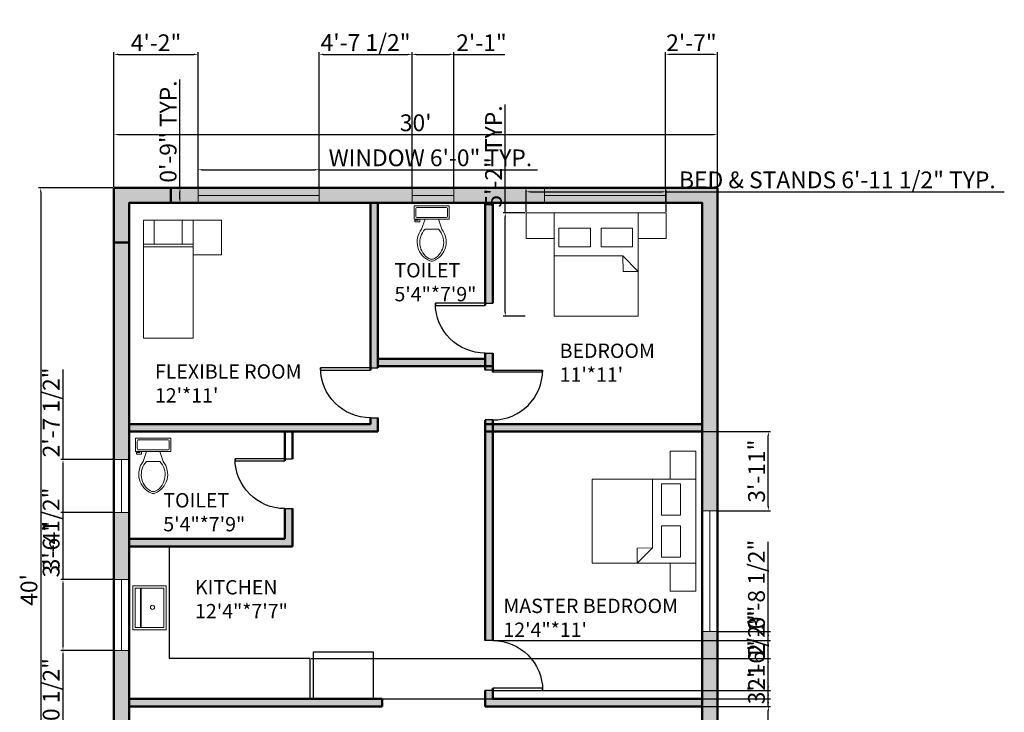
# Model space of a CAD drawing. Units: inches. Extents: x 1369 to 1956, y 3714 to 4363.
# Tile 2 of 2: x 1369 to 1956, y 3949 to 4363. Entities that reach past the tile are written whole.
import ezdxf

# ---------------------------------------------------------------- set-up
doc = ezdxf.new("R2010")
doc.units = ezdxf.units.IN
for name, color, linetype, lineweight in [('A-ANNO-DIMS', 2, 'Continuous', 18), ('A-AREA-IDEN', 7, 'Continuous', 25), ('A-DOOR', 3, 'Continuous', 25), ('A-FLOR-CASE', 9, 'Continuous', 25), ('A-FLOR-FIXT', 9, 'Continuous', 18), ('A-FURN', 8, 'Continuous', 18), ('A-GLAZ', 4, 'Continuous', 18), ('A-WALL', 7, 'Continuous', 50), ('A-WALL-PATT', 252, 'Continuous', 13)]:
    doc.layers.add(name, color=color, linetype=linetype, lineweight=lineweight)
doc.styles.get("Standard").update_dxf_attribs({"font": 'arial.ttf'})
doc.dimstyles.new('ISO-25', dxfattribs={"dimtxt": 10, "dimasz": 2.5, "dimexe": 1.25, "dimexo": 0.625, "dimtad": 1, "dimdec": 0, "dimlunit": 4, "dimtxsty": 'Standard', "dimcen": 2.5, "dimadec": 0, "dimazin": 0, "dimtfac": 1, "dimtdec": 0, "dimtmove": 0, "dimatfit": 3, "dimfxl": 1, "dimarcsym": 0})

# ---------------------------------------------------------------- blocks, each defined once
blk = doc.blocks.new('*U2')
for p, q in [((0, 0), (0, -6)), ((40, 0), (40, -6))]:
    blk.add_line(p, q)
blk.add_lwpolyline([(0, 0), (0, 40), (1.75, 40), (1.75, 0)], close=True)
blk.add_arc((0, 0), 40, 0, 90)
blk = doc.blocks.new('*U4')
for p, q in [((9.5, -6), (9.5, -2)), ((-10, -8.5), (-8, -8.5)), ((-10, -9.5), (-10, -8.5)), ((-7, -9.5), (-10, -9.5)), ((-8, -8.5), (-8, -8)), ((-7, -8), (-7, -9.5)), ((-4, -8), (-6, -14)), ((4, -8), (6, -14)), ((4, -14), (-4, -14))]:
    blk.add_line(p, q)
blk.add_lwpolyline([(10.5, -8), (10.5, 0), (-10.5, 0), (-10.5, -8)], close=True)
for points in [[(-9.5, -2), (-9.5, -6)], [(8.5, -1), (-8.5, -1)], [(-8.5, -7), (8.5, -7)]]:
    blk.add_lwpolyline(points)
for centre, radius, start, end in [((-8.62, -1.88), 0.884, 81.8699, 188.1301), ((8.62, -1.88), 0.884, 351.8699, 98.1301), ((-8.62, -6.12), 0.884, 171.8699, 278.1301), ((8.62, -6.12), 0.884, 261.8699, 8.1301), ((3.52, -21.58), 12.17, 141.46911, 247.97143), ((4.2, -21.82), 11.33, 136.36773, 238.94682), ((-3.52, -21.58), 12.17, 292.02843, 38.53071), ((-4.2, -21.82), 11.33, 301.05301, 43.63209), ((0, -27.88), 4, 245.73182, 294.26817), ((0, -29), 4, 254.86053, 285.13947)]:
    blk.add_arc(centre, radius, start, end)
blk = doc.blocks.new('*D5')
at = {"layer": 'A-ANNO-DIMS', "color": 0, "lineweight": -2, "transparency": 16777216}
for p, q in [((1425.18, 4263.07), (1425.18, 4295.53)), ((1427.68, 4294.28), (1782.68, 4294.28)), ((1785.18, 4263.07), (1785.18, 4295.53))]:
    blk.add_line(p, q, dxfattribs=at)
at = {"layer": 'A-ANNO-DIMS', "color": 0, "transparency": 16777216}
for points in [[(1427.68, 4294.69), (1427.68, 4293.86), (1425.18, 4294.28)], [(1782.68, 4294.69), (1782.68, 4293.86), (1785.18, 4294.28)]]:
    blk.add_solid(points, dxfattribs=at)
at = {"layer": 'Defpoints', "color": 0, "transparency": 16777216}
for p in [(1785.18, 4294.28), (1425.18, 4262.45), (1785.18, 4262.45)]:
    blk.add_point(p, dxfattribs=at)
at = {"layer": 'A-ANNO-DIMS', "color": 0, "transparency": 16777216, "insert": (1605.18, 4300.01), "char_height": 10, "attachment_point": 5}
blk.add_mtext("30'", dxfattribs=at)
blk = doc.blocks.new('*D6')
at = {"layer": 'A-ANNO-DIMS', "color": 0, "lineweight": -2, "transparency": 16777216}
for p, q in [((1424.56, 4262.45), (1380.24, 4262.45)), ((1381.49, 4259.95), (1381.49, 3784.95)), ((1424.56, 3782.45), (1380.24, 3782.45))]:
    blk.add_line(p, q, dxfattribs=at)
at = {"layer": 'A-ANNO-DIMS', "color": 0, "transparency": 16777216}
for points in [[(1381.07, 4259.95), (1381.9, 4259.95), (1381.49, 4262.45)], [(1381.07, 3784.95), (1381.9, 3784.95), (1381.49, 3782.45)]]:
    blk.add_solid(points, dxfattribs=at)
at = {"layer": 'Defpoints', "color": 0, "transparency": 16777216}
for p in [(1425.18, 4262.45), (1381.49, 3782.45), (1425.18, 3782.45)]:
    blk.add_point(p, dxfattribs=at)
at = {"layer": 'A-ANNO-DIMS', "color": 0, "transparency": 16777216, "insert": (1375.76, 4022.45), "char_height": 10, "attachment_point": 5, "rotation": 90}
blk.add_mtext("40'", dxfattribs=at)
blk = doc.blocks.new('BED-DOUBLE-WITH-NIGHTSTANDS')
for p, q in [((16.69, 36.1), (57.66, 36.1)), ((57.66, 36.1), (66.84, 26.79)), ((57.8, 26.79), (57.66, 36.1)), ((66.84, 26.79), (57.8, 26.79))]:
    blk.add_line(p, q)
for points in [[(0, 61.8), (16.69, 61.8), (16.69, 46.54), (0, 46.54)], [(16.69, 61.8), (66.84, 61.8), (66.84, 0), (16.69, 0)], [(66.84, 61.8), (83.53, 61.8), (83.53, 46.54), (66.84, 46.54)], [(19.52, 52.7), (38.23, 52.7), (38.23, 41.44), (19.52, 41.44)], [(44.61, 52.7), (63.32, 52.7), (63.32, 41.44), (44.61, 41.44)]]:
    blk.add_lwpolyline(points, close=True)
blk = doc.blocks.new('WINDOW-72IN')
blk.add_line((0, 4.5), (72.22, 4.5))
blk.add_lwpolyline([(0, 9), (72.22, 9), (72.22, 0), (0, 0)], close=True)
blk = doc.blocks.new('*D10')
at = {"layer": 'A-ANNO-DIMS', "color": 0, "lineweight": -2, "transparency": 16777216}
for p, q in [((1475.37, 4263.07), (1475.37, 4274.53)), ((1477.87, 4273.28), (1545.09, 4273.28)), ((1547.59, 4263.07), (1547.59, 4274.53)), ((1547.59, 4273.28), (1677.88, 4273.28))]:
    blk.add_line(p, q, dxfattribs=at)
at = {"layer": 'A-ANNO-DIMS', "color": 0, "transparency": 16777216}
for points in [[(1477.87, 4273.7), (1477.87, 4272.86), (1475.37, 4273.28)], [(1545.09, 4273.7), (1545.09, 4272.86), (1547.59, 4273.28)]]:
    blk.add_solid(points, dxfattribs=at)
at = {"layer": 'Defpoints', "color": 0, "transparency": 16777216}
for p in [(1547.59, 4273.28), (1475.37, 4262.45), (1547.59, 4262.45)]:
    blk.add_point(p, dxfattribs=at)
at = {"layer": 'A-ANNO-DIMS', "color": 0, "transparency": 16777216, "insert": (1613.98, 4279.08), "char_height": 10, "attachment_point": 5}
blk.add_mtext('WINDOW 6\'-0" TYP.', dxfattribs=at)
blk = doc.blocks.new('*D11')
at = {"layer": 'A-ANNO-DIMS', "color": 0, "lineweight": -2, "transparency": 16777216}
for p, q in [((1464.54, 4262.45), (1464.54, 4327.15)), ((1474.74, 4262.45), (1463.29, 4262.45)), ((1464.54, 4255.95), (1464.54, 4259.95)), ((1474.74, 4253.45), (1463.29, 4253.45))]:
    blk.add_line(p, q, dxfattribs=at)
at = {"layer": 'A-ANNO-DIMS', "color": 0, "transparency": 16777216}
for points in [[(1464.12, 4259.95), (1464.95, 4259.95), (1464.54, 4262.45)], [(1464.12, 4255.95), (1464.95, 4255.95), (1464.54, 4253.45)]]:
    blk.add_solid(points, dxfattribs=at)
at = {"layer": 'Defpoints', "color": 0, "transparency": 16777216}
for p in [(1464.54, 4262.45), (1475.37, 4262.45), (1475.37, 4253.45)]:
    blk.add_point(p, dxfattribs=at)
at = {"layer": 'A-ANNO-DIMS', "color": 0, "transparency": 16777216, "insert": (1458.81, 4296.05), "char_height": 10, "attachment_point": 5, "rotation": 90}
blk.add_mtext('0\'-9" TYP.', dxfattribs=at)
blk = doc.blocks.new('*D14')
at = {"layer": 'A-ANNO-DIMS', "color": 0, "lineweight": -2, "transparency": 16777216}
for p, q in [((1671.16, 4248.19), (1671.16, 4261.34)), ((1673.66, 4260.09), (1752.18, 4260.09)), ((1754.68, 4248.19), (1754.68, 4261.34)), ((1754.68, 4260.09), (1956.37, 4260.09))]:
    blk.add_line(p, q, dxfattribs=at)
at = {"layer": 'A-ANNO-DIMS', "color": 0, "transparency": 16777216}
for points in [[(1673.66, 4260.51), (1673.66, 4259.67), (1671.16, 4260.09)], [(1752.18, 4260.51), (1752.18, 4259.67), (1754.68, 4260.09)]]:
    blk.add_solid(points, dxfattribs=at)
at = {"layer": 'Defpoints', "color": 0, "transparency": 16777216}
for p in [(1754.68, 4260.09), (1671.16, 4247.56), (1754.68, 4247.56)]:
    blk.add_point(p, dxfattribs=at)
at = {"layer": 'A-ANNO-DIMS', "color": 0, "transparency": 16777216, "insert": (1856.78, 4265.92), "char_height": 10, "attachment_point": 5}
blk.add_mtext('BED & STANDS 6\'-11 1/2" TYP.', dxfattribs=at)
blk = doc.blocks.new('*D15')
at = {"layer": 'A-ANNO-DIMS', "color": 0, "lineweight": -2, "transparency": 16777216}
for p, q in [((1658.63, 4247.56), (1658.63, 4312.27)), ((1670.53, 4247.56), (1657.38, 4247.56)), ((1658.63, 4188.27), (1658.63, 4245.06)), ((1670.53, 4185.77), (1657.38, 4185.77))]:
    blk.add_line(p, q, dxfattribs=at)
at = {"layer": 'A-ANNO-DIMS', "color": 0, "transparency": 16777216}
for points in [[(1658.21, 4245.06), (1659.04, 4245.06), (1658.63, 4247.56)], [(1658.21, 4188.27), (1659.04, 4188.27), (1658.63, 4185.77)]]:
    blk.add_solid(points, dxfattribs=at)
at = {"layer": 'Defpoints', "color": 0, "transparency": 16777216}
for p in [(1658.63, 4247.56), (1671.16, 4247.56), (1671.16, 4185.77)]:
    blk.add_point(p, dxfattribs=at)
at = {"layer": 'A-ANNO-DIMS', "color": 0, "transparency": 16777216, "insert": (1652.9, 4281.16), "char_height": 10, "attachment_point": 5, "rotation": 90}
blk.add_mtext('5\'-2" TYP.', dxfattribs=at)
blk = doc.blocks.new('*D21')
at = {"layer": 'A-ANNO-DIMS', "color": 0, "lineweight": -2, "transparency": 16777216}
for p, q in [((1425.18, 4263.07), (1425.18, 4343.38)), ((1427.68, 4342.13), (1472.87, 4342.13)), ((1475.37, 4263.07), (1475.37, 4343.38))]:
    blk.add_line(p, q, dxfattribs=at)
at = {"layer": 'A-ANNO-DIMS', "color": 0, "transparency": 16777216}
for points in [[(1427.68, 4342.55), (1427.68, 4341.71), (1425.18, 4342.13)], [(1472.87, 4342.55), (1472.87, 4341.71), (1475.37, 4342.13)]]:
    blk.add_solid(points, dxfattribs=at)
at = {"layer": 'Defpoints', "color": 0, "transparency": 16777216}
for p in [(1475.37, 4342.13), (1425.18, 4262.45), (1475.37, 4262.45)]:
    blk.add_point(p, dxfattribs=at)
at = {"layer": 'A-ANNO-DIMS', "color": 0, "transparency": 16777216, "insert": (1450.28, 4347.77), "char_height": 10, "attachment_point": 5}
blk.add_mtext('4\'-2"', dxfattribs=at)
blk = doc.blocks.new('*D22')
at = {"layer": 'A-ANNO-DIMS', "color": 0, "lineweight": -2, "transparency": 16777216}
for p, q in [((1754.24, 4263.07), (1754.24, 4343.38)), ((1782.68, 4342.13), (1756.74, 4342.13)), ((1785.18, 4263.07), (1785.18, 4343.38))]:
    blk.add_line(p, q, dxfattribs=at)
at = {"layer": 'A-ANNO-DIMS', "color": 0, "transparency": 16777216}
for points in [[(1756.74, 4342.55), (1756.74, 4341.71), (1754.24, 4342.13)], [(1782.68, 4342.55), (1782.68, 4341.71), (1785.18, 4342.13)]]:
    blk.add_solid(points, dxfattribs=at)
at = {"layer": 'Defpoints', "color": 0, "transparency": 16777216}
for p in [(1754.24, 4342.13), (1754.24, 4262.45), (1785.18, 4262.45)]:
    blk.add_point(p, dxfattribs=at)
at = {"layer": 'A-ANNO-DIMS', "color": 0, "transparency": 16777216, "insert": (1769.71, 4347.77), "char_height": 10, "attachment_point": 5}
blk.add_mtext('2\'-7"', dxfattribs=at)
blk = doc.blocks.new('*D26')
at = {"layer": 'A-ANNO-DIMS', "color": 0, "lineweight": -2, "transparency": 16777216}
for p, q in [((1815.58, 3952.95), (1815.58, 4006.57)), ((1776.81, 3952.95), (1816.83, 3952.95)), ((1815.58, 3917.75), (1815.58, 3950.45)), ((1785.81, 3915.25), (1816.83, 3915.25))]:
    blk.add_line(p, q, dxfattribs=at)
at = {"layer": 'A-ANNO-DIMS', "color": 0, "transparency": 16777216}
for points in [[(1815.16, 3950.45), (1816, 3950.45), (1815.58, 3952.95)], [(1815.16, 3917.75), (1816, 3917.75), (1815.58, 3915.25)]]:
    blk.add_solid(points, dxfattribs=at)
at = {"layer": 'Defpoints', "color": 0, "transparency": 16777216}
for p in [(1776.18, 3952.95), (1815.58, 3952.95), (1785.18, 3915.25)]:
    blk.add_point(p, dxfattribs=at)
at = {"layer": 'A-ANNO-DIMS', "color": 0, "transparency": 16777216, "insert": (1809.78, 3981.01), "char_height": 10, "attachment_point": 5, "rotation": 90}
blk.add_mtext('3\'-1 1/2"', dxfattribs=at)
blk = doc.blocks.new('*D27')
at = {"layer": 'A-ANNO-DIMS', "color": 0, "lineweight": -2, "transparency": 16777216}
for p, q in [((1815.58, 3997.53), (1815.58, 4051.16)), ((1785.81, 3997.53), (1816.83, 3997.53)), ((1815.58, 3955.45), (1815.58, 3995.03)), ((1776.81, 3952.95), (1816.83, 3952.95))]:
    blk.add_line(p, q, dxfattribs=at)
at = {"layer": 'A-ANNO-DIMS', "color": 0, "transparency": 16777216}
for points in [[(1815.16, 3995.03), (1816, 3995.03), (1815.58, 3997.53)], [(1815.16, 3955.45), (1816, 3955.45), (1815.58, 3952.95)]]:
    blk.add_solid(points, dxfattribs=at)
at = {"layer": 'Defpoints', "color": 0, "transparency": 16777216}
for p in [(1785.18, 3997.53), (1815.58, 3997.53), (1776.18, 3952.95)]:
    blk.add_point(p, dxfattribs=at)
at = {"layer": 'A-ANNO-DIMS', "color": 0, "transparency": 16777216, "insert": (1809.78, 4025.6), "char_height": 10, "attachment_point": 5, "rotation": 90}
blk.add_mtext('3\'-8 1/2"', dxfattribs=at)
blk = doc.blocks.new('*D28')
at = {"layer": 'A-ANNO-DIMS', "color": 0, "lineweight": -2, "transparency": 16777216}
for p, q in [((1776.81, 4116.95), (1816.83, 4116.95)), ((1815.58, 4072.25), (1815.58, 4114.45)), ((1785.81, 4069.75), (1816.83, 4069.75))]:
    blk.add_line(p, q, dxfattribs=at)
at = {"layer": 'A-ANNO-DIMS', "color": 0, "transparency": 16777216}
for points in [[(1815.16, 4114.45), (1816, 4114.45), (1815.58, 4116.95)], [(1815.16, 4072.25), (1816, 4072.25), (1815.58, 4069.75)]]:
    blk.add_solid(points, dxfattribs=at)
at = {"layer": 'Defpoints', "color": 0, "transparency": 16777216}
for p in [(1776.18, 4116.95), (1815.58, 4116.95), (1785.18, 4069.75)]:
    blk.add_point(p, dxfattribs=at)
at = {"layer": 'A-ANNO-DIMS', "color": 0, "transparency": 16777216, "insert": (1809.85, 4093.35), "char_height": 10, "attachment_point": 5, "rotation": 90}
blk.add_mtext('3\'-11"', dxfattribs=at)
blk = doc.blocks.new('*D29')
at = {"layer": 'A-ANNO-DIMS', "color": 0, "lineweight": -2, "transparency": 16777216}
for p, q in [((1394.78, 4028.64), (1394.78, 4082.27)), ((1424.56, 4028.64), (1393.53, 4028.64)), ((1394.78, 3988.85), (1394.78, 4026.14)), ((1424.56, 3986.35), (1393.53, 3986.35))]:
    blk.add_line(p, q, dxfattribs=at)
at = {"layer": 'A-ANNO-DIMS', "color": 0, "transparency": 16777216}
for points in [[(1394.36, 4026.14), (1395.2, 4026.14), (1394.78, 4028.64)], [(1394.36, 3988.85), (1395.2, 3988.85), (1394.78, 3986.35)]]:
    blk.add_solid(points, dxfattribs=at)
at = {"layer": 'Defpoints', "color": 0, "transparency": 16777216}
for p in [(1394.78, 4028.64), (1425.18, 4028.64), (1425.18, 3986.35)]:
    blk.add_point(p, dxfattribs=at)
at = {"layer": 'A-ANNO-DIMS', "color": 0, "transparency": 16777216, "insert": (1388.98, 4056.71), "char_height": 10, "attachment_point": 5, "rotation": 90}
blk.add_mtext('3\'-6 1/2"', dxfattribs=at)
blk = doc.blocks.new('*D30')
at = {"layer": 'A-ANNO-DIMS', "color": 0, "lineweight": -2, "transparency": 16777216}
for p, q in [((1394.78, 4100.25), (1394.78, 4154.05)), ((1424.56, 4100.25), (1393.53, 4100.25)), ((1394.78, 4071.11), (1394.78, 4097.75)), ((1424.56, 4068.61), (1393.53, 4068.61))]:
    blk.add_line(p, q, dxfattribs=at)
at = {"layer": 'A-ANNO-DIMS', "color": 0, "transparency": 16777216}
for points in [[(1394.36, 4097.75), (1395.2, 4097.75), (1394.78, 4100.25)], [(1394.36, 4071.11), (1395.2, 4071.11), (1394.78, 4068.61)]]:
    blk.add_solid(points, dxfattribs=at)
at = {"layer": 'Defpoints', "color": 0, "transparency": 16777216}
for p in [(1394.78, 4100.25), (1425.18, 4100.25), (1425.18, 4068.61)]:
    blk.add_point(p, dxfattribs=at)
at = {"layer": 'A-ANNO-DIMS', "color": 0, "transparency": 16777216, "insert": (1388.99, 4128.4), "char_height": 10, "attachment_point": 5, "rotation": 90}
blk.add_mtext('2\'-7 1/2"', dxfattribs=at)
blk = doc.blocks.new('*D31')
at = {"layer": 'A-ANNO-DIMS', "color": 0, "lineweight": -2, "transparency": 16777216}
for p, q in [((1424.56, 4068.61), (1393.53, 4068.61)), ((1394.78, 4031.14), (1394.78, 4066.11)), ((1424.56, 4028.64), (1393.53, 4028.64))]:
    blk.add_line(p, q, dxfattribs=at)
at = {"layer": 'A-ANNO-DIMS', "color": 0, "transparency": 16777216}
for points in [[(1394.36, 4066.11), (1395.2, 4066.11), (1394.78, 4068.61)], [(1394.36, 4031.14), (1395.2, 4031.14), (1394.78, 4028.64)]]:
    blk.add_solid(points, dxfattribs=at)
at = {"layer": 'Defpoints', "color": 0, "transparency": 16777216}
for p in [(1394.78, 4068.61), (1425.18, 4068.61), (1425.18, 4028.64)]:
    blk.add_point(p, dxfattribs=at)
at = {"layer": 'A-ANNO-DIMS', "color": 0, "transparency": 16777216, "insert": (1389.05, 4048.63), "char_height": 10, "attachment_point": 5, "rotation": 90}
blk.add_mtext('3\'-4"', dxfattribs=at)
blk = doc.blocks.new('*D32')
at = {"layer": 'A-ANNO-DIMS', "color": 0, "lineweight": -2, "transparency": 16777216}
for p, q in [((1424.56, 3986.35), (1393.53, 3986.35)), ((1394.78, 3918.43), (1394.78, 3983.85)), ((1433.56, 3915.93), (1393.53, 3915.93))]:
    blk.add_line(p, q, dxfattribs=at)
at = {"layer": 'A-ANNO-DIMS', "color": 0, "transparency": 16777216}
for points in [[(1394.36, 3983.85), (1395.2, 3983.85), (1394.78, 3986.35)], [(1394.36, 3918.43), (1395.2, 3918.43), (1394.78, 3915.93)]]:
    blk.add_solid(points, dxfattribs=at)
at = {"layer": 'Defpoints', "color": 0, "transparency": 16777216}
for p in [(1394.78, 3986.35), (1425.18, 3986.35), (1434.18, 3915.93)]:
    blk.add_point(p, dxfattribs=at)
at = {"layer": 'A-ANNO-DIMS', "color": 0, "transparency": 16777216, "insert": (1388.99, 3951.14), "char_height": 10, "attachment_point": 5, "rotation": 90}
blk.add_mtext('5\'-10 1/2"', dxfattribs=at)
blk = doc.blocks.new('*D33')
at = {"layer": 'A-ANNO-DIMS', "color": 0, "lineweight": -2, "transparency": 16777216}
for p, q in [((1603.01, 4263.07), (1603.01, 4343.38)), ((1605.51, 4342.13), (1625.44, 4342.13)), ((1627.94, 4263.07), (1627.94, 4343.38)), ((1627.94, 4342.13), (1658.44, 4342.13))]:
    blk.add_line(p, q, dxfattribs=at)
at = {"layer": 'A-ANNO-DIMS', "color": 0, "transparency": 16777216}
for points in [[(1605.51, 4342.55), (1605.51, 4341.71), (1603.01, 4342.13)], [(1625.44, 4342.55), (1625.44, 4341.71), (1627.94, 4342.13)]]:
    blk.add_solid(points, dxfattribs=at)
at = {"layer": 'Defpoints', "color": 0, "transparency": 16777216}
for p in [(1627.94, 4342.13), (1603.01, 4262.45), (1627.94, 4262.45)]:
    blk.add_point(p, dxfattribs=at)
at = {"layer": 'A-ANNO-DIMS', "color": 0, "transparency": 16777216, "insert": (1644.44, 4347.77), "char_height": 10, "attachment_point": 5}
blk.add_mtext('2\'-1"', dxfattribs=at)
blk = doc.blocks.new('*D34')
at = {"layer": 'A-ANNO-DIMS', "color": 0, "lineweight": -2, "transparency": 16777216}
for p, q in [((1547.59, 4263.07), (1547.59, 4343.38)), ((1550.09, 4342.13), (1600.51, 4342.13)), ((1603.01, 4263.07), (1603.01, 4343.38))]:
    blk.add_line(p, q, dxfattribs=at)
at = {"layer": 'A-ANNO-DIMS', "color": 0, "transparency": 16777216}
for points in [[(1550.09, 4342.55), (1550.09, 4341.71), (1547.59, 4342.13)], [(1600.51, 4342.55), (1600.51, 4341.71), (1603.01, 4342.13)]]:
    blk.add_solid(points, dxfattribs=at)
at = {"layer": 'Defpoints', "color": 0, "transparency": 16777216}
for p in [(1603.01, 4342.13), (1547.59, 4262.45), (1603.01, 4262.45)]:
    blk.add_point(p, dxfattribs=at)
at = {"layer": 'A-ANNO-DIMS', "color": 0, "transparency": 16777216, "insert": (1575.3, 4347.92), "char_height": 10, "attachment_point": 5}
blk.add_mtext('4\'-7 1/2"', dxfattribs=at)
blk = doc.blocks.new('*D35')
at = {"layer": 'A-ANNO-DIMS', "color": 0, "lineweight": -2, "transparency": 16777216}
for p, q in [((1651.81, 3992.23), (1816.83, 3992.23)), ((1815.58, 3964.95), (1815.58, 3989.73)), ((1651.77, 3962.45), (1816.83, 3962.45))]:
    blk.add_line(p, q, dxfattribs=at)
at = {"layer": 'A-ANNO-DIMS', "color": 0, "transparency": 16777216}
for points in [[(1815.16, 3989.73), (1816, 3989.73), (1815.58, 3992.23)], [(1815.16, 3964.95), (1816, 3964.95), (1815.58, 3962.45)]]:
    blk.add_solid(points, dxfattribs=at)
at = {"layer": 'Defpoints', "color": 0, "transparency": 16777216}
for p in [(1651.18, 3992.23), (1815.58, 3992.23), (1651.15, 3962.45)]:
    blk.add_point(p, dxfattribs=at)
at = {"layer": 'A-ANNO-DIMS', "color": 0, "transparency": 16777216, "insert": (1809.85, 3977.34), "char_height": 10, "attachment_point": 5, "rotation": 90}
blk.add_mtext('2\'-6"', dxfattribs=at)
blk = doc.blocks.new('*D36')
at = {"layer": 'A-ANNO-DIMS', "color": 0, "lineweight": -2, "transparency": 16777216}
for p, q in [((1815.58, 3981.45), (1815.58, 4011.95)), ((1542.78, 3981.45), (1816.83, 3981.45)), ((1815.58, 3959.95), (1815.58, 3978.95)), ((1542.78, 3957.45), (1816.83, 3957.45))]:
    blk.add_line(p, q, dxfattribs=at)
at = {"layer": 'A-ANNO-DIMS', "color": 0, "transparency": 16777216}
for points in [[(1815.16, 3978.95), (1816, 3978.95), (1815.58, 3981.45)], [(1815.16, 3959.95), (1816, 3959.95), (1815.58, 3957.45)]]:
    blk.add_solid(points, dxfattribs=at)
at = {"layer": 'Defpoints', "color": 0, "transparency": 16777216}
for p in [(1542.15, 3981.45), (1815.58, 3981.45), (1542.15, 3957.45)]:
    blk.add_point(p, dxfattribs=at)
at = {"layer": 'A-ANNO-DIMS', "color": 0, "transparency": 16777216, "insert": (1809.85, 3997.95), "char_height": 10, "attachment_point": 5, "rotation": 90}
blk.add_mtext('2\'-0"', dxfattribs=at)

msp = doc.modelspace()

# ---------------------------------------------------------------- hatches: boundary and pattern name
at = {"layer": 'A-WALL-PATT'}
h = msp.add_hatch(color=256, dxfattribs=at)
h.dxf.hatch_style = 1
h.paths.add_polyline_path([(1785.18, 3997.53), (1776.18, 3997.53), (1776.18, 3915.25), (1785.18, 3915.25)])
h.paths.add_polyline_path([(1776.18, 3957.45), (1651.18, 3957.45), (1651.18, 3962.45), (1651.15, 3962.45), (1646.68, 3962.45), (1646.68, 3957.45), (1646.68, 3952.95), (1776.18, 3952.95)], flags=17)
h.paths.add_polyline_path([(1651.18, 4116.95), (1646.68, 4116.95), (1646.68, 3992.23), (1651.18, 3992.23)])
h.paths.add_polyline_path([(1585.18, 3957.45), (1434.18, 3957.45), (1434.18, 3952.95), (1582.18, 3952.95), (1585.18, 3952.95)], flags=17)
h.paths.add_polyline_path([(1434.18, 3986.35), (1425.18, 3986.35), (1425.18, 3782.45), (1785.18, 3782.45), (1785.18, 3843.04), (1776.18, 3843.04), (1776.18, 3791.45), (1434.18, 3791.45)])
h.paths.add_polyline_path([(1531.68, 4070.96), (1527.18, 4070.96), (1527.18, 4052.95), (1434.18, 4052.95), (1434.18, 4048.45), (1531.68, 4048.45)])
h.paths.add_polyline_path([(1434.18, 4048.45), (1434.18, 4052.95), (1434.18, 4068.61), (1425.18, 4068.61), (1425.18, 4028.64), (1434.18, 4028.64)])
h.paths.add_polyline_path([(1785.18, 4262.45), (1425.18, 4262.45), (1425.18, 4100.25), (1434.18, 4100.25), (1434.18, 4116.95), (1434.18, 4253.45), (1776.18, 4253.45), (1776.18, 4069.75), (1785.18, 4069.75)])
h.paths.add_polyline_path([(1776.18, 4121.45), (1651.18, 4121.45), (1651.18, 4116.95), (1776.18, 4116.95)], flags=17)
h.paths.add_polyline_path([(1651.18, 4121.45), (1646.68, 4121.45), (1646.68, 4116.95), (1651.18, 4116.95)], flags=17)
h.paths.add_polyline_path([(1582.68, 4125.18), (1578.18, 4125.18), (1578.18, 4121.45), (1434.18, 4121.45), (1434.18, 4116.95), (1582.68, 4116.95)], flags=17)
h.paths.add_polyline_path([(1582.68, 4253.45), (1578.18, 4253.45), (1578.18, 4154.96), (1578.21, 4154.96), (1582.68, 4154.96)], flags=17)
h.paths.add_polyline_path([(1651.18, 4253.45), (1646.68, 4253.45), (1646.68, 4193.53), (1646.71, 4193.53), (1651.18, 4193.53)], flags=17)
h.paths.add_polyline_path([(1646.68, 4160.45), (1582.68, 4160.45), (1582.68, 4155.95), (1646.68, 4155.95)], flags=17)
h.paths.add_polyline_path([(1651.18, 4163.74), (1646.68, 4163.74), (1646.68, 4160.45), (1646.68, 4155.95), (1651.18, 4155.95)], flags=17)
h.paths.add_polyline_path([(1651.18, 4123.87), (1646.68, 4123.87), (1646.68, 4121.45), (1651.18, 4121.45)], flags=17)
h.paths.add_polyline_path([(1651.18, 4155.95), (1646.68, 4155.95), (1646.68, 4153.66), (1651.18, 4153.66)], flags=17)
h.paths.add_polyline_path([(1515.18, 3904.98), (1515.18, 3915.93), (1506.18, 3915.93), (1506.18, 3894.63), (1506.18, 3791.45), (1515.18, 3791.45)], flags=17)

# ---------------------------------------------------------------- linework, layer by layer
at = {"layer": 'A-FLOR-CASE'}
for p, q in [((1434.18, 4048.45), (1434.18, 4024.45)), ((1434.18, 4048.45), (1458.18, 4048.45)), ((1458.18, 4048.45), (1458.18, 3981.45)), ((1542.15, 3981.45), (1458.18, 3981.45)), ((1542.15, 3957.45), (1542.15, 3981.45))]:
    msp.add_line(p, q, dxfattribs=at)
msp.add_lwpolyline([(1579.81, 3957.45), (1544.29, 3957.45), (1544.29, 3985.46), (1579.81, 3985.46)], close=True, dxfattribs=at)
at = {"layer": 'A-FLOR-FIXT'}
for p, q in [((1440.98, 4023.55), (1440.98, 4000.04)), ((1441.42, 4023.55), (1441.42, 4000.04))]:
    msp.add_line(p, q, dxfattribs=at)
for points in [[(1436.4, 3998.7), (1456.26, 3998.7), (1456.26, 4024.9), (1436.4, 4024.9)], [(1437.75, 4000.04), (1454.92, 4000.04), (1454.92, 4023.55), (1437.75, 4023.55)]]:
    msp.add_lwpolyline(points, close=True, dxfattribs=at)
msp.add_circle((1448.16, 4012.04), 1.24, dxfattribs=at)
at = {"layer": 'A-FURN'}
for points in [[(1442.88, 4243.2), (1472.39, 4243.2), (1472.39, 4172.77), (1442.88, 4172.77)], [(1449.26, 4228.92), (1465.86, 4228.92), (1465.86, 4243.2), (1449.26, 4243.2)], [(1472.39, 4243.2), (1489.37, 4243.2), (1489.37, 4222.55), (1472.39, 4222.55)], [(1472.39, 4228.92), (1442.88, 4228.92), (1442.88, 4227.33), (1472.39, 4227.33)]]:
    msp.add_lwpolyline(points, close=True, dxfattribs=at)
at = {"layer": 'A-GLAZ'}
for p, q in [((1603.01, 4257.95), (1627.94, 4257.95)), ((1429.68, 4068.61), (1429.68, 4100.25)), ((1429.68, 3986.35), (1429.68, 4028.64))]:
    msp.add_line(p, q, dxfattribs=at)
for points in [[(1603.01, 4253.45), (1627.94, 4253.45), (1627.94, 4262.45), (1603.01, 4262.45)], [(1434.18, 4100.25), (1425.18, 4100.25), (1425.18, 4068.61), (1434.18, 4068.61)], [(1434.18, 4028.64), (1425.18, 4028.64), (1425.18, 3986.35), (1434.18, 3986.35)]]:
    msp.add_lwpolyline(points, close=True, dxfattribs=at)
at = {"layer": 'A-WALL'}
for p, q in [((1459.1, 4253.45), (1459.1, 4262.45)), ((1434.18, 4253.45), (1578.18, 4253.45)), ((1578.18, 4253.45), (1578.18, 4153.66)), ((1582.68, 4253.45), (1582.68, 4154.96)), ((1582.68, 4253.45), (1646.68, 4253.45)), ((1646.68, 4253.45), (1646.68, 4192.22)), ((1651.18, 4253.45), (1651.18, 4193.53)), ((1776.18, 4253.45), (1776.18, 4121.45)), ((1434.18, 4229.93), (1425.18, 4229.93)), ((1646.68, 4160.45), (1582.68, 4160.45)), ((1646.68, 4163.74), (1646.68, 4160.45)), ((1646.68, 4160.45), (1646.68, 4155.95)), ((1651.18, 4163.74), (1651.18, 4155.95)), ((1651.18, 4155.95), (1582.68, 4155.95)), ((1646.68, 4155.95), (1646.68, 4153.66)), ((1651.18, 4155.95), (1651.18, 4152.35)), ((1578.18, 4125.18), (1578.18, 4121.45)), ((1582.68, 4125.18), (1582.68, 4116.95)), ((1646.68, 4123.87), (1646.68, 4116.95)), ((1651.18, 4123.87), (1651.18, 4116.95)), ((1578.18, 4121.45), (1434.18, 4121.45)), ((1446.18, 4121.45), (1434.18, 4121.45)), ((1776.18, 4121.45), (1646.68, 4121.45)), ((1582.68, 4116.95), (1434.18, 4116.95)), ((1434.18, 4116.95), (1434.18, 4052.95)), ((1527.18, 4099.43), (1527.18, 4116.95)), ((1531.68, 4100.74), (1531.68, 4116.95)), ((1776.18, 4116.95), (1646.68, 4116.95)), ((1646.68, 4116.95), (1646.68, 3992.23)), ((1651.18, 4116.95), (1651.18, 3992.23)), ((1527.18, 4052.95), (1527.18, 4070.96)), ((1531.68, 4048.45), (1531.68, 4070.96)), ((1434.18, 4052.95), (1527.18, 4052.95)), ((1434.18, 4048.45), (1531.68, 4048.45)), ((1434.18, 4048.45), (1434.18, 3957.45)), ((1646.68, 3962.45), (1646.68, 3957.45)), ((1651.18, 3963.75), (1651.18, 3957.45)), ((1434.18, 3957.45), (1582.18, 3957.45)), ((1434.18, 3957.45), (1585.18, 3957.45)), ((1582.18, 3957.45), (1585.18, 3957.45)), ((1585.18, 3957.45), (1585.18, 3952.95)), ((1646.68, 3957.45), (1646.68, 3952.95)), ((1651.18, 3957.45), (1776.18, 3957.45)), ((1434.18, 3952.95), (1582.18, 3952.95)), ((1582.18, 3952.95), (1585.18, 3952.95)), ((1646.68, 3952.95), (1776.18, 3952.95))]:
    msp.add_line(p, q, dxfattribs=at)
for points in [[(1425.18, 3782.45), (1785.18, 3782.45), (1785.18, 4262.45), (1425.18, 4262.45)], [(1434.18, 3791.45), (1776.18, 3791.45), (1776.18, 4253.45), (1434.18, 4253.45)]]:
    msp.add_lwpolyline(points, close=True, dxfattribs=at)

# ---------------------------------------------------------------- block references
at = {"layer": 'A-DOOR', "yscale": 0.744547159397362, "zscale": 0.744547159397362}
for p, xscale, rotation in [((1646.71, 4193.53), -0.744547159397362, 90), ((1578.21, 4154.96), -0.744547159397362, 90), ((1651.15, 4153.66), 0.744547159397362, 270), ((1527.21, 4100.74), -0.744547159397362, 90), ((1651.15, 3962.45), -0.744547159397362, 270)]:
    msp.add_blockref('*U2', p, dxfattribs=dict(at, xscale=xscale, rotation=rotation))
at = {"layer": 'A-FLOR-FIXT'}
for p in [(1614.76, 4251.73), (1448.6, 4113.06)]:
    msp.add_blockref('*U4', p, dxfattribs=at)
at = {"layer": 'A-FURN'}
msp.add_blockref('BED-DOUBLE-WITH-NIGHTSTANDS', (1671.16, 4185.77), dxfattribs=at)
at = {"layer": 'A-FURN', "rotation": 269.9999999999993}
msp.add_blockref('BED-DOUBLE-WITH-NIGHTSTANDS', (1710.47, 4105.25), dxfattribs=at)
at = {"layer": 'A-GLAZ'}
for p in [(1475.37, 4253.45), (1682.02, 4253.45)]:
    msp.add_blockref('WINDOW-72IN', p, dxfattribs=at)
at = {"layer": 'A-GLAZ', "rotation": 269.9999999999997}
msp.add_blockref('WINDOW-72IN', (1776.18, 4069.75), dxfattribs=at)

# ---------------------------------------------------------------- texts
at = {"layer": 'A-AREA-IDEN', "attachment_point": 1}
for s, insert, char_height in [('TOILET\\P5\'4"*7\'9"', (1592.53, 4217.54), 8.55), ("BEDROOM\\P11'*11'", (1691.11, 4169.47), 8.55), ("FLEXIBLE ROOM\\P12'*11'", (1449.65, 4157.1), 8.5497), ('TOILET\\P5\'4"*7\'9"', (1454.63, 4080.23), 8.55), ('KITCHEN\\P12\'4"*7\'7"', (1473.56, 4028.32), 8.55), ('MASTER BEDROOM\\P12\'4"*11\'', (1657.53, 4017.2), 8.5497)]:
    msp.add_mtext_dynamic_manual_height_columns(s, width=219.0068, gutter_width=42.75, heights=[0], dxfattribs=dict(at, insert=insert, char_height=char_height))

# ---------------------------------------------------------------- dimensions: what is measured, and where the dimension line sits
at = {"layer": 'A-ANNO-DIMS'}
for base, p1, p2, override, picture, middle in [((1603.01, 4342.13), (1547.59, 4262.45), (1603.01, 4262.45), {"dimdec": 1, "dimlfac": 1, "dimrnd": 0, "dimzin": 1, "dimdsep": 46, "dimlunit": 4, "dimfrac": 2}, '*D34', (1575.3, 4347.92)), ((1475.37, 4342.13), (1425.18, 4262.45), (1475.37, 4262.45), {"dimdec": 1, "dimlfac": 1, "dimrnd": 0, "dimzin": 1, "dimdsep": 46, "dimlunit": 4, "dimfrac": 2}, '*D21', (1450.28, 4347.77)), ((1627.94, 4342.13), (1603.01, 4262.45), (1627.94, 4262.45), {"dimdec": 1, "dimlfac": 1, "dimrnd": 0, "dimzin": 1, "dimdsep": 46, "dimlunit": 4, "dimfrac": 2}, '*D33', (1644.44, 4347.77)), ((1754.24, 4342.13), (1785.18, 4262.45), (1754.24, 4262.45), {"dimdec": 1, "dimlfac": 1, "dimrnd": 0, "dimzin": 1, "dimdsep": 46, "dimlunit": 4, "dimfrac": 2}, '*D22', (1769.71, 4347.77)), ((1785.18, 4294.28), (1425.18, 4262.45), (1785.18, 4262.45), {"dimclrd": 0, "dimclre": 0, "dimclrt": 0}, '*D5', (1605.18, 4300.01))]:
    dim = msp.add_linear_dim(base=base, p1=p1, p2=p2, dimstyle='ISO-25', override=override, dxfattribs=at)
    dim.commit()
    dim.dimension.update_dxf_attribs({"geometry": picture, "text_midpoint": middle})
for base, p1, p2, picture, middle in [((1464.54, 4262.45), (1475.37, 4253.45), (1475.37, 4262.45), '*D11', (1458.81, 4296.05)), ((1658.63, 4247.56), (1671.16, 4185.77), (1671.16, 4247.56), '*D15', (1652.9, 4281.16))]:
    dim = msp.add_linear_dim(base=base, p1=p1, p2=p2, angle=90, text='<> TYP.', dimstyle='ISO-25', override={"dimdec": 1, "dimlfac": 1, "dimrnd": 0, "dimzin": 1, "dimdsep": 46, "dimlunit": 4, "dimfrac": 2}, dxfattribs=at)
    dim.commit()
    dim.dimension.update_dxf_attribs({"geometry": picture, "text_midpoint": middle})
for base, p1, p2, text, picture, middle in [((1754.68, 4260.09), (1671.16, 4247.56), (1754.68, 4247.56), 'BED & STANDS <> TYP.', '*D14', (1856.78, 4265.92)), ((1547.59, 4273.28), (1475.37, 4262.45), (1547.59, 4262.45), 'WINDOW <> TYP.', '*D10', (1613.98, 4279.08))]:
    dim = msp.add_linear_dim(base=base, p1=p1, p2=p2, text=text, dimstyle='ISO-25', override={"dimdec": 1, "dimlfac": 1, "dimrnd": 0, "dimzin": 1, "dimdsep": 46, "dimlunit": 4, "dimfrac": 2}, dxfattribs=at)
    dim.commit()
    dim.dimension.update_dxf_attribs({"geometry": picture, "text_midpoint": middle})
for base, p1, p2, override, picture, middle in [((1381.49, 3782.45), (1425.18, 4262.45), (1425.18, 3782.45), {"dimclrd": 0, "dimclre": 0, "dimclrt": 0}, '*D6', (1375.76, 4022.45)), ((1394.78, 4100.25), (1425.18, 4068.61), (1425.18, 4100.25), {"dimdec": 1, "dimlfac": 1, "dimrnd": 0, "dimzin": 1, "dimdsep": 46, "dimlunit": 4, "dimfrac": 2}, '*D30', (1388.99, 4128.4)), ((1815.58, 4116.95), (1785.18, 4069.75), (1776.18, 4116.95), {"dimdec": 1, "dimlfac": 1, "dimrnd": 0, "dimzin": 1, "dimdsep": 46, "dimlunit": 4, "dimfrac": 2}, '*D28', (1809.85, 4093.35)), ((1394.78, 4028.64), (1425.18, 3986.35), (1425.18, 4028.64), {"dimdec": 1, "dimlfac": 1, "dimrnd": 0, "dimzin": 1, "dimdsep": 46, "dimlunit": 4, "dimfrac": 2}, '*D29', (1388.98, 4056.71)), ((1394.78, 4068.61), (1425.18, 4028.64), (1425.18, 4068.61), {"dimdec": 1, "dimlfac": 1, "dimrnd": 0, "dimzin": 1, "dimdsep": 46, "dimlunit": 4, "dimfrac": 2}, '*D31', (1389.05, 4048.63)), ((1815.58, 3997.53), (1776.18, 3952.95), (1785.18, 3997.53), {"dimdec": 1, "dimlfac": 1, "dimrnd": 0, "dimzin": 1, "dimdsep": 46, "dimlunit": 4, "dimfrac": 2}, '*D27', (1809.78, 4025.6)), ((1815.58, 3981.45), (1542.15, 3957.45), (1542.15, 3981.45), {"dimdec": 1, "dimlfac": 1, "dimrnd": 0, "dimzin": 1, "dimdsep": 46, "dimlunit": 4, "dimfrac": 2}, '*D36', (1809.85, 3997.95)), ((1815.58, 3952.95), (1785.18, 3915.25), (1776.18, 3952.95), {"dimdec": 1, "dimlfac": 1, "dimrnd": 0, "dimzin": 1, "dimdsep": 46, "dimlunit": 4, "dimfrac": 2}, '*D26', (1809.78, 3981.01)), ((1815.58, 3992.23), (1651.15, 3962.45), (1651.18, 3992.23), {"dimdec": 1, "dimlfac": 1, "dimrnd": 0, "dimzin": 1, "dimdsep": 46, "dimlunit": 4, "dimfrac": 2}, '*D35', (1809.85, 3977.34)), ((1394.78, 3986.35), (1434.18, 3915.93), (1425.18, 3986.35), {"dimdec": 1, "dimlfac": 1, "dimrnd": 0, "dimzin": 1, "dimdsep": 46, "dimlunit": 4, "dimfrac": 2}, '*D32', (1388.99, 3951.14))]:
    dim = msp.add_linear_dim(base=base, p1=p1, p2=p2, angle=90, dimstyle='ISO-25', override=override, dxfattribs=at)
    dim.commit()
    dim.dimension.update_dxf_attribs({"geometry": picture, "text_midpoint": middle})

doc.saveas('drawing.dxf')
